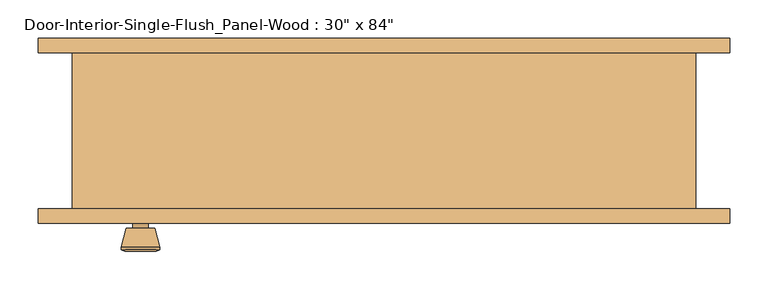
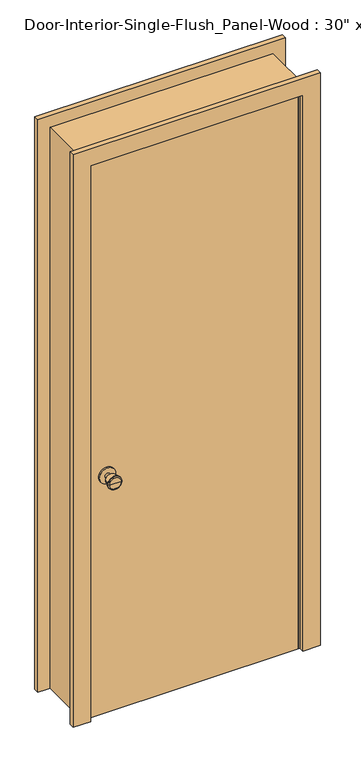
"""IFC4 building model written with IfcOpenShell, lengths in millimetres: door geometry."""

from ifc_helpers import new_model, si_unit, point, frame, frame_2d, origin, origin_with_axes, place, context, project, spatial, polyline, circle_curve, trimmed, segment, composite_curve, outline, extrude, faceted_brep, source, transform, mapped, element, save
from ifc_brep_helpers import plane_surface, cylinder_surface, revolved_surface, advanced_brep


def door_701f8457(model_context):
    return source(origin(), model_context, "Body", "SolidModel", [
        advanced_brep(
        [(-317.5, -57.5, 914.4), (-327.5, -57.5, 914.4), (-307.5, -57.5, 914.4), (-297.0241324, -8.5, 914.4), (-337.9758676, -8.5, 914.4), (-317.5, -8.5, 914.4), (-292.5, -10.3278681, 914.4), (-342.5, -10.3278681, 914.4), (-292.5, -13.7915463, 914.4), (-342.5, -13.7915463, 914.4), (-298.863764, -38.5, 914.4), (-336.136236, -38.5, 914.4), (-307.5, -38.5, 914.4), (-327.5, -38.5, 914.4)],
        [
            (0, 1),
            (1, 2, circle_curve(frame((-317.5, -57.5, 914.4), z_axis=(0.0, -1.0, 0.0), x_axis=(-1.0, 0.0, 0.0)), 10.0)),
            (2, 0),
            (2, 1, circle_curve(frame((-317.5, -57.5, 914.4), z_axis=(0.0, -1.0, 0.0), x_axis=(-1.0, 0.0, 0.0)), 10.0)),
            (3, 4, circle_curve(frame((-317.5, -8.5, 914.4), z_axis=(0.0, 1.0, 0.0), x_axis=(-1.0, 0.0, 0.0)), 20.4758676)),
            (4, 5),
            (5, 3),
            (4, 3, circle_curve(frame((-317.5, -8.5, 914.4), z_axis=(0.0, 1.0, 0.0), x_axis=(-1.0, 0.0, 0.0)), 20.4758676)),
            (6, 7, circle_curve(frame((-317.5, -10.3278681, 914.4), z_axis=(0.0, 1.0, 0.0), x_axis=(-1.0, 0.0, 0.0)), 25.0)),
            (7, 4),
            (3, 6),
            (7, 6, circle_curve(frame((-317.5, -10.3278681, 914.4), z_axis=(0.0, 1.0, 0.0), x_axis=(-1.0, 0.0, 0.0)), 25.0)),
            (8, 9, circle_curve(frame((-317.5, -13.7915463, 914.4), z_axis=(0.0, 1.0, 0.0), x_axis=(-1.0, 0.0, 0.0)), 25.0)),
            (9, 7),
            (6, 8),
            (9, 8, circle_curve(frame((-317.5, -13.7915463, 914.4), z_axis=(0.0, 1.0, 0.0), x_axis=(-1.0, 0.0, 0.0)), 25.0)),
            (10, 11, circle_curve(frame((-317.5, -38.5, 914.4), z_axis=(0.0, 1.0, 0.0), x_axis=(-1.0, 0.0, 0.0)), 18.636236)),
            (11, 9),
            (8, 10),
            (11, 10, circle_curve(frame((-317.5, -38.5, 914.4), z_axis=(0.0, 1.0, 0.0), x_axis=(-1.0, 0.0, 0.0)), 18.636236)),
            (12, 13, circle_curve(frame((-317.5, -38.5, 914.4), z_axis=(0.0, 1.0, 0.0), x_axis=(-1.0, 0.0, 0.0)), 10.0)),
            (13, 11),
            (10, 12),
            (13, 12, circle_curve(frame((-317.5, -38.5, 914.4), z_axis=(0.0, 1.0, 0.0), x_axis=(-1.0, 0.0, 0.0)), 10.0)),
            (1, 13),
            (12, 2),
        ],
        [
            plane_surface(frame((-317.5, -57.5, 914.4), z_axis=(0.0, -1.0, 0.0), x_axis=(-1.0, 0.0, 0.0))),
            plane_surface(frame((-317.5, -8.5, 914.4), z_axis=(0.0, 1.0, 0.0), x_axis=(-1.0, 0.0, 0.0))),
            revolved_surface(polyline([(-337.9758676, -8.5, 914.4), (-342.5, -10.3278681, 914.4)]), (-317.5, -57.5, 914.4), (0.0, -1.0, 0.0)),
            cylinder_surface(frame((-317.5, -57.5, 914.4), z_axis=(0.0, -1.0, 0.0), x_axis=(-1.0, 0.0, 0.0)), 25.0),
            revolved_surface(polyline([(-342.5, -13.7915463, 914.4), (-336.136236, -38.5, 914.4)]), (-317.5, -57.5, 914.4), (0.0, -1.0, 0.0)),
            plane_surface(frame((-317.5, -38.5, 914.4), z_axis=(0.0, -1.0, 0.0), x_axis=(-1.0, 0.0, 0.0))),
            cylinder_surface(frame((-317.5, -57.5, 914.4), z_axis=(0.0, -1.0, 0.0), x_axis=(-1.0, 0.0, 0.0)), 10.0),
        ],
        [
            (0, [[1, 2, 3]]),
            (0, [[-3, 4, -1]]),
            (1, [[5, 6, 7]]),
            (1, [[8, -7, -6]]),
            (2, [[9, 10, -5, 11]]),
            (2, [[12, -11, -8, -10]]),
            (3, [[13, 14, -9, 15]]),
            (3, [[16, -15, -12, -14]]),
            (4, [[17, 18, -13, 19]]),
            (4, [[20, -19, -16, -18]]),
            (5, [[21, 22, -17, 23]]),
            (5, [[24, -23, -20, -22]]),
            (6, [[-2, 25, -21, 26]]),
            (6, [[-4, -26, -24, -25]]),
        ],
    ),
        extrude(outline(composite_curve([segment(trimmed(circle_curve(frame_2d((914.4, -317.5)), 30.0), [point((914.4, -347.5))], [point((914.4, -287.5))], False, "CARTESIAN"), True, "CONTINUOUS"), segment(trimmed(circle_curve(frame_2d((914.4, -317.5)), 30.0), [point((914.4, -287.5))], [point((914.4, -347.5))], False, "CARTESIAN"), True, "CONTINUOUS")], self_intersect=False)), frame((0.0, -63.5, 0.0), z_axis=(0.0, 1.0, 0.0), x_axis=(0.0, 0.0, 1.0)), (0.0, 0.0, 1.0), 6.0),
        advanced_brep(
        [(-317.5, -104.425, 914.4), (-307.5, -104.425, 914.4), (-327.5, -104.425, 914.4), (-297.0241324, -153.425, 914.4), (-317.5, -153.425, 914.4), (-337.9758676, -153.425, 914.4), (-292.5, -151.5971319, 914.4), (-342.5, -151.5971319, 914.4), (-292.5, -148.1334537, 914.4), (-342.5, -148.1334537, 914.4), (-298.863764, -123.425, 914.4), (-336.136236, -123.425, 914.4), (-307.5, -123.425, 914.4), (-327.5, -123.425, 914.4)],
        [
            (0, 1),
            (1, 2, circle_curve(frame((-317.5, -104.425, 914.4), z_axis=(0.0, 1.0, 0.0), x_axis=(-1.0, 0.0, 0.0)), 10.0)),
            (2, 0),
            (2, 1, circle_curve(frame((-317.5, -104.425, 914.4), z_axis=(0.0, 1.0, 0.0), x_axis=(-1.0, 0.0, 0.0)), 10.0)),
            (3, 4),
            (4, 5),
            (5, 3, circle_curve(frame((-317.5, -153.425, 914.4), z_axis=(0.0, -1.0, 0.0), x_axis=(-1.0, 0.0, 0.0)), 20.4758676)),
            (3, 5, circle_curve(frame((-317.5, -153.425, 914.4), z_axis=(0.0, -1.0, 0.0), x_axis=(-1.0, 0.0, 0.0)), 20.4758676)),
            (6, 3),
            (5, 7),
            (7, 6, circle_curve(frame((-317.5, -151.5971319, 914.4), z_axis=(0.0, -1.0, 0.0), x_axis=(-1.0, 0.0, 0.0)), 25.0)),
            (6, 7, circle_curve(frame((-317.5, -151.5971319, 914.4), z_axis=(0.0, -1.0, 0.0), x_axis=(-1.0, 0.0, 0.0)), 25.0)),
            (8, 6),
            (7, 9),
            (9, 8, circle_curve(frame((-317.5, -148.1334537, 914.4), z_axis=(0.0, -1.0, 0.0), x_axis=(-1.0, 0.0, 0.0)), 25.0)),
            (8, 9, circle_curve(frame((-317.5, -148.1334537, 914.4), z_axis=(0.0, -1.0, 0.0), x_axis=(-1.0, 0.0, 0.0)), 25.0)),
            (10, 8),
            (9, 11),
            (11, 10, circle_curve(frame((-317.5, -123.425, 914.4), z_axis=(0.0, -1.0, 0.0), x_axis=(-1.0, 0.0, 0.0)), 18.636236)),
            (10, 11, circle_curve(frame((-317.5, -123.425, 914.4), z_axis=(0.0, -1.0, 0.0), x_axis=(-1.0, 0.0, 0.0)), 18.636236)),
            (12, 10),
            (11, 13),
            (13, 12, circle_curve(frame((-317.5, -123.425, 914.4), z_axis=(0.0, -1.0, 0.0), x_axis=(-1.0, 0.0, 0.0)), 10.0)),
            (12, 13, circle_curve(frame((-317.5, -123.425, 914.4), z_axis=(0.0, -1.0, 0.0), x_axis=(-1.0, 0.0, 0.0)), 10.0)),
            (1, 12),
            (13, 2),
        ],
        [
            plane_surface(frame((-317.5, -104.425, 914.4), z_axis=(0.0, 1.0, 0.0), x_axis=(-1.0, 0.0, 0.0))),
            plane_surface(frame((-317.5, -153.425, 914.4), z_axis=(0.0, -1.0, 0.0), x_axis=(-1.0, 0.0, 0.0))),
            revolved_surface(polyline([(-337.9758676, -153.425, 914.4), (-342.5, -151.5971319, 914.4)]), (-317.5, -104.425, 914.4), (0.0, 1.0, 0.0)),
            cylinder_surface(frame((-317.5, -104.425, 914.4), z_axis=(0.0, 1.0, 0.0), x_axis=(-1.0, 0.0, 0.0)), 25.0),
            revolved_surface(polyline([(-342.5, -148.1334537, 914.4), (-336.136236, -123.425, 914.4)]), (-317.5, -104.425, 914.4), (0.0, 1.0, 0.0)),
            plane_surface(frame((-317.5, -123.425, 914.4), z_axis=(0.0, 1.0, 0.0), x_axis=(-1.0, 0.0, 0.0))),
            cylinder_surface(frame((-317.5, -104.425, 914.4), z_axis=(0.0, 1.0, 0.0), x_axis=(-1.0, 0.0, 0.0)), 10.0),
        ],
        [
            (0, [[1, 2, 3]]),
            (0, [[-3, 4, -1]]),
            (1, [[5, 6, 7]]),
            (1, [[-6, -5, 8]]),
            (2, [[9, -7, 10, 11]]),
            (2, [[-10, -8, -9, 12]]),
            (3, [[13, -11, 14, 15]]),
            (3, [[-14, -12, -13, 16]]),
            (4, [[17, -15, 18, 19]]),
            (4, [[-18, -16, -17, 20]]),
            (5, [[21, -19, 22, 23]]),
            (5, [[-22, -20, -21, 24]]),
            (6, [[25, -23, 26, -2]]),
            (6, [[-26, -24, -25, -4]]),
        ],
    ),
        extrude(outline(composite_curve([segment(trimmed(circle_curve(frame_2d((914.4, -317.5)), 30.0), [point((914.4, -347.5))], [point((914.4, -287.5))], False, "CARTESIAN"), True, "CONTINUOUS"), segment(trimmed(circle_curve(frame_2d((914.4, -317.5)), 30.0), [point((914.4, -287.5))], [point((914.4, -347.5))], False, "CARTESIAN"), True, "CONTINUOUS")], self_intersect=False)), frame((0.0, -104.425, 0.0), z_axis=(0.0, 1.0, 0.0), x_axis=(0.0, 0.0, 1.0)), (0.0, 0.0, 1.0), 6.0),
        extrude(outline(polyline([(381.0, -63.5), (381.0, -98.425), (-381.0, -98.425), (-381.0, -63.5), (381.0, -63.5)])), origin_with_axes(), (0.0, 0.0, 1.0), 2133.6),
        faceted_brep([(406.4, -98.425, 0.0), (381.0, -98.425, 0.0), (381.0, -63.5, 0.0), (368.3, -63.5, 0.0), (368.3, -28.575, 0.0), (381.0, -28.575, 0.0), (381.0, 104.775, 0.0), (406.4, 104.775, 0.0), (406.4, 104.775, 2159.0), (406.4, -98.425, 2159.0), (381.0, 104.775, 2133.6), (-381.0, 104.775, 2133.6), (-381.0, 104.775, 0.0), (-406.4, 104.775, 0.0), (-406.4, 104.775, 2159.0), (381.0, -28.575, 2133.6), (368.3, -28.575, 2120.9), (-368.3, -28.575, 2120.9), (-368.3, -28.575, 0.0), (-381.0, -28.575, 0.0), (-381.0, -28.575, 2133.6), (368.3, -63.5, 2120.9), (381.0, -63.5, 2133.6), (-381.0, -63.5, 2133.6), (-381.0, -63.5, 0.0), (-368.3, -63.5, 0.0), (-368.3, -63.5, 2120.9), (381.0, -98.425, 2133.6), (-406.4, -98.425, 2159.0), (-406.4, -98.425, 0.0), (-381.0, -98.425, 0.0), (-381.0, -98.425, 2133.6)], [[[0, 1, 2, 3, 4, 5, 6, 7]], [[7, 8, 9, 0]], [[6, 10, 11, 12, 13, 14, 8, 7]], [[5, 15, 10, 6]], [[4, 16, 17, 18, 19, 20, 15, 5]], [[3, 21, 16, 4]], [[2, 22, 23, 24, 25, 26, 21, 3]], [[1, 27, 22, 2]], [[0, 9, 28, 29, 30, 31, 27, 1]], [[8, 14, 28, 9]], [[15, 20, 11, 10]], [[21, 26, 17, 16]], [[27, 31, 23, 22]], [[29, 13, 12, 19, 18, 25, 24, 30]], [[14, 13, 29, 28]], [[20, 19, 12, 11]], [[26, 25, 18, 17]], [[31, 30, 24, 23]]]),
        extrude(outline(polyline([(0.0, 450.85), (2203.45, 450.85), (2203.45, -450.85), (0.0, -450.85), (0.0, -387.35), (2139.95, -387.35), (2139.95, 387.35), (0.0, 387.35), (0.0, 450.85)])), frame((0.0, 104.775, 0.0), z_axis=(0.0, 1.0, 0.0), x_axis=(0.0, 0.0, 1.0)), (0.0, 0.0, 1.0), 19.05),
        extrude(outline(polyline([(0.0, 450.85), (2203.45, 450.85), (2203.45, -450.85), (0.0, -450.85), (0.0, -387.35), (2139.95, -387.35), (2139.95, 387.35), (0.0, 387.35), (0.0, 450.85)])), frame((0.0, -117.475, 0.0), z_axis=(0.0, 1.0, 0.0), x_axis=(0.0, 0.0, 1.0)), (0.0, 0.0, 1.0), 19.05),
    ])


if __name__ == "__main__":
    model = new_model("IFC4")
    model_context = context("Model", 3, world=origin())
    ifc_project = project(units=[si_unit("LENGTHUNIT", "METRE", prefix="MILLI")], contexts=[model_context])
    site = spatial("IfcSite", under=ifc_project)
    building = spatial("IfcBuilding", under=site)
    placement = place(None, origin())
    door_shape = door_701f8457(model_context)
    element("IfcDoor", 1, ObjectType="Door-Interior-Single-Flush_Panel-Wood : 30\" x 84\"", at=placement, inside=building, context=model_context, shape_type="MappedRepresentation", body=[
        mapped(door_shape, transform((0.0, 0.0, 0.0), x_axis=(1.0, 0.0, 0.0), y_axis=(0.0, 1.0, 0.0), z_axis=(0.0, 0.0, 1.0))),
    ])
    save(model, "model.ifc")

# Revit data of these elements
# Type "Door-Interior-Single-Flush_Panel-Wood : 30\" x 84\""
#   Type Mark = "12"
#   Assembly Code = "C1020300"
#   Analytic Construction = "Wooden"
#   Thickness = 0' - 1 3/8"
#   Thermal Resistance (R) = 2.5876 (h·ft²·°F)/BTU
#   Swing Angle [instance default] = 90.00°
#   Rough Width = 2' - 8"
#   Rough Height = 7' - 1"
#   Height = 7' - 0"
#   Width = 2' - 6"
#   Heat Transfer Coefficient (U) = 0.3865 BTU/(h·ft²·°F)
#   Trim Material = Cherry
#   Panel Material = Cherry
#   Frame Material = Cherry
#   Door Handle Material = Aluminum
#   Visual Light Transmittance = 0
#   Solar Heat Gain Coefficient = 0
#   Wall Closure = (empty or 0)
#   Function = (empty or 0)
# Element 1 (IfcDoor, "Door-Interior-Single-Flush_Panel-Wood : 30\" x 84\"")
#   Materials on its faces: "Cherry", "Aluminum"
# Materials
#   "Cherry": class "Wood", colour RGB 226 177 128, transparency 0, Description = "Prunus Serotina", Cost = 0
#   "Aluminum": class "Metal", colour RGB 247 247 247, transparency 0, Description = "Aluminum 6061", Cost = 0
